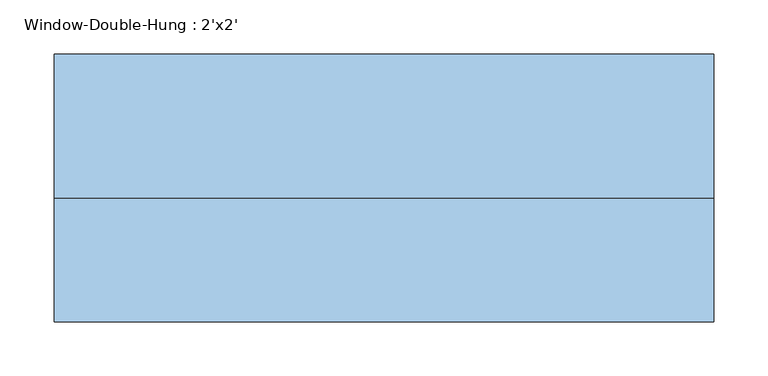
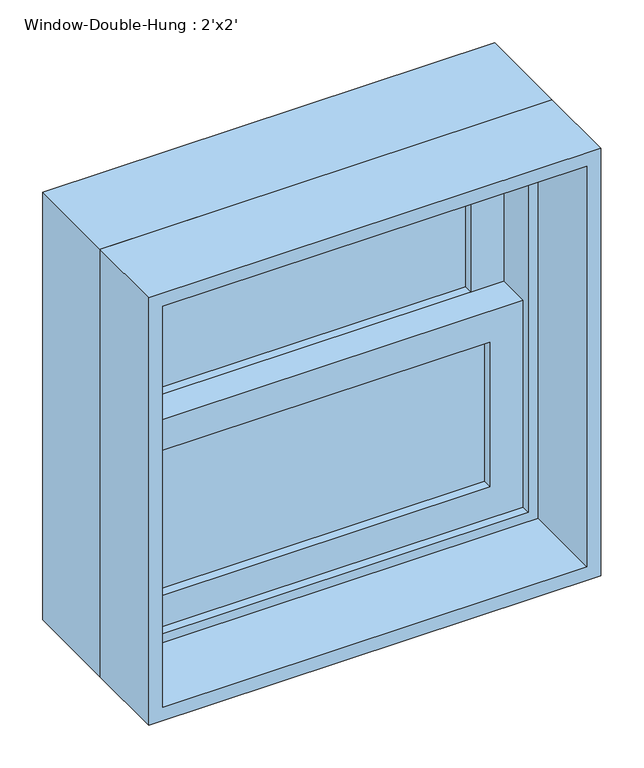
"""IFC4 building model written with IfcOpenShell, lengths in millimetres: window geometry, Window-Double-Hung : 2'x2'."""

from ifc_helpers import new_model, si_unit, frame, origin, place, context, project, spatial, polyline, outline, extrude, source, transform, mapped, element, save


def window_double_hung_2_x2_15b2d83c(model_context):
    return source(origin(), model_context, "Body", "SweptSolid", [
        extrude(outline(polyline([(228.6, 44.45), (228.6, 38.1), (-228.6, 38.1), (-228.6, 44.45), (228.6, 44.45)])), frame((0.0, 0.0, 990.6), z_axis=(0.0, 0.0, 1.0), x_axis=(1.0, 0.0, 0.0)), (0.0, 0.0, 1.0), 206.375),
        extrude(outline(polyline([(-228.6, 31.75), (228.6, 31.75), (228.6, 25.4), (-228.6, 25.4), (-228.6, 31.75)])), frame((0.0, 0.0, 990.6), z_axis=(0.0, 0.0, 1.0), x_axis=(1.0, 0.0, 0.0)), (0.0, 0.0, 1.0), 206.375),
        extrude(outline(polyline([(228.6, 88.9), (228.6, 82.55), (-228.6, 82.55), (-228.6, 88.9), (228.6, 88.9)])), frame((0.0, 0.0, 1241.425), z_axis=(0.0, 0.0, 1.0), x_axis=(1.0, 0.0, 0.0)), (0.0, 0.0, 1.0), 206.375),
        extrude(outline(polyline([(-228.6, 76.2), (228.6, 76.2), (228.6, 69.85), (-228.6, 69.85), (-228.6, 76.2)])), frame((0.0, 0.0, 1241.425), z_axis=(0.0, 0.0, 1.0), x_axis=(1.0, 0.0, 0.0)), (0.0, 0.0, 1.0), 206.375),
        extrude(outline(polyline([(1241.425, -273.05), (946.15, -273.05), (946.15, 273.05), (1241.425, 273.05), (1241.425, -273.05)]), holes=[polyline([(1196.975, 228.6), (990.6, 228.6), (990.6, -228.6), (1196.975, -228.6), (1196.975, 228.6)])]), frame((0.0, 12.7, 0.0), z_axis=(0.0, 1.0, 0.0), x_axis=(0.0, 0.0, 1.0)), (0.0, 0.0, 1.0), 44.45),
        extrude(outline(polyline([(1492.25, -273.05), (1196.975, -273.05), (1196.975, 273.05), (1492.25, 273.05), (1492.25, -273.05)]), holes=[polyline([(1447.8, 228.6), (1241.425, 228.6), (1241.425, -228.6), (1447.8, -228.6), (1447.8, 228.6)])]), frame((0.0, 57.15, 0.0), z_axis=(0.0, 1.0, 0.0), x_axis=(0.0, 0.0, 1.0)), (0.0, 0.0, 1.0), 44.45),
        extrude(outline(polyline([(1524.0, -304.8), (914.4, -304.8), (914.4, 304.8), (1524.0, 304.8), (1524.0, -304.8)]), holes=[polyline([(1492.25, 273.05), (946.15, 273.05), (946.15, -273.05), (1492.25, -273.05), (1492.25, 273.05)])]), frame((0.0, 0.0, 0.0), z_axis=(0.0, 1.0, 0.0), x_axis=(0.0, 0.0, 1.0)), (0.0, 0.0, 1.0), 133.35),
        extrude(outline(polyline([(1524.0, 304.8), (1524.0, -304.8), (914.4, -304.8), (914.4, 304.8), (1524.0, 304.8)]), holes=[polyline([(1504.95, 285.75), (933.45, 285.75), (933.45, -285.75), (1504.95, -285.75), (1504.95, 285.75)])]), frame((0.0, -114.3, 0.0), z_axis=(0.0, 1.0, 0.0), x_axis=(0.0, 0.0, 1.0)), (0.0, 0.0, 1.0), 114.3),
    ])


if __name__ == "__main__":
    model = new_model("IFC4")
    model_context = context("Model", 3, world=origin())
    ifc_project = project(units=[si_unit("LENGTHUNIT", "METRE", prefix="MILLI")], contexts=[model_context])
    site = spatial("IfcSite", under=ifc_project)
    building = spatial("IfcBuilding", under=site)
    placement = place(None, origin())
    window_double_hung_2_x2_shape = window_double_hung_2_x2_15b2d83c(model_context)
    element("IfcWindow", 1, ObjectType="Window-Double-Hung : 2'x2'", at=placement, inside=building, context=model_context, shape_type="MappedRepresentation", body=[
        mapped(window_double_hung_2_x2_shape, transform((0.0, 0.0, 0.0), x_axis=(1.0, 0.0, 0.0), y_axis=(0.0, 1.0, 0.0), z_axis=(0.0, 0.0, 1.0))),
    ])
    save(model, "model.ifc")

# Revit data of these elements
# Type "Window-Double-Hung : 2'x2'"
#   Type Mark = "26"
#   Fire Rating = "0.5h"
#   Construction Type Id = "DG-DR"
#   Assembly Code = "B2020100"
#   Analytic Construction = "Double glazing - domestic"
#   Wall Thickness [instance default] = 0' - 6"
#   Window Inset [instance default] = 0' - 0"
#   Visual Light Transmittance = 0.81
#   Thermal Resistance (R) = 1.8146 (h·ft²·°F)/BTU
#   Solar Heat Gain Coefficient = 0.76
#   Muntin Width = 1' - 6"
#   Muntin Height = 0' - 8 1/8"
#   Interior Wall Closure [instance default] = 0' - 1 1/2"
#   Rough Width = 2' - 0 1/2"
#   Rough Height = 2' - 0 1/2"
#   Frame Extension [instance default] = 0' - 1 1/4"
#   Exterior Wall Closure [instance default] = 0' - 0 1/2"
#   Extension Jamb [instance default] = 0' - 1 1/2"
#   Heat Transfer Coefficient (U) = 0.5511 BTU/(h·ft²·°F)
#   Height = 2' - 0"
#   Width = 2' - 0"
#   Top Muntin Visibility = yes
#   Indicator Visibility [instance default] = yes
#   Extension Jamb Visibility [instance default] = yes
#   Interior Trim Visibility [instance default] = yes
#   Exterior Trim Visibility [instance default] = yes
#   Define Thermal Properties by = 1
#   Bottom Muntin Visibility = yes
#   Muntin Pattern = Muntin Pattern_2x2 : Muntin Pattern_2x2
#   Interior Trim Material = Wood - Stained
#   Interior Trim = Trim-Window-Interior-Flat : Picture Frame
#   Exterior Trim Material = Clad - White
#   Exterior Trim = Trim-Window-Exterior-Flat : with Sill
#   Glass Panel Material = Glass
#   Exterior Frame Material = Clad - White
#   Interior Frame Material = Wood - Stained
#   Wall Closure = (empty or 0)
# Element 1 (IfcWindow, "Window-Double-Hung : 2'x2'")
#   Wall Thickness = 0' - 9"
#   Extension Jamb = 0' - 4 1/2"
#   Materials on its faces: "Wood - Stained", "Glass", "Clad - White"
# Materials
#   "Wood - Stained": class "Wood", colour RGB 224 178 126, transparency 0, Cost = 0
#   "Clad - White": class "Wood", colour RGB 242 242 238, transparency 0, Cost = 0
#   "Glass": class "Glass", colour RGB 154 182 205, transparency 0.85, Description = "Soda Lime Glass", Cost = 0
